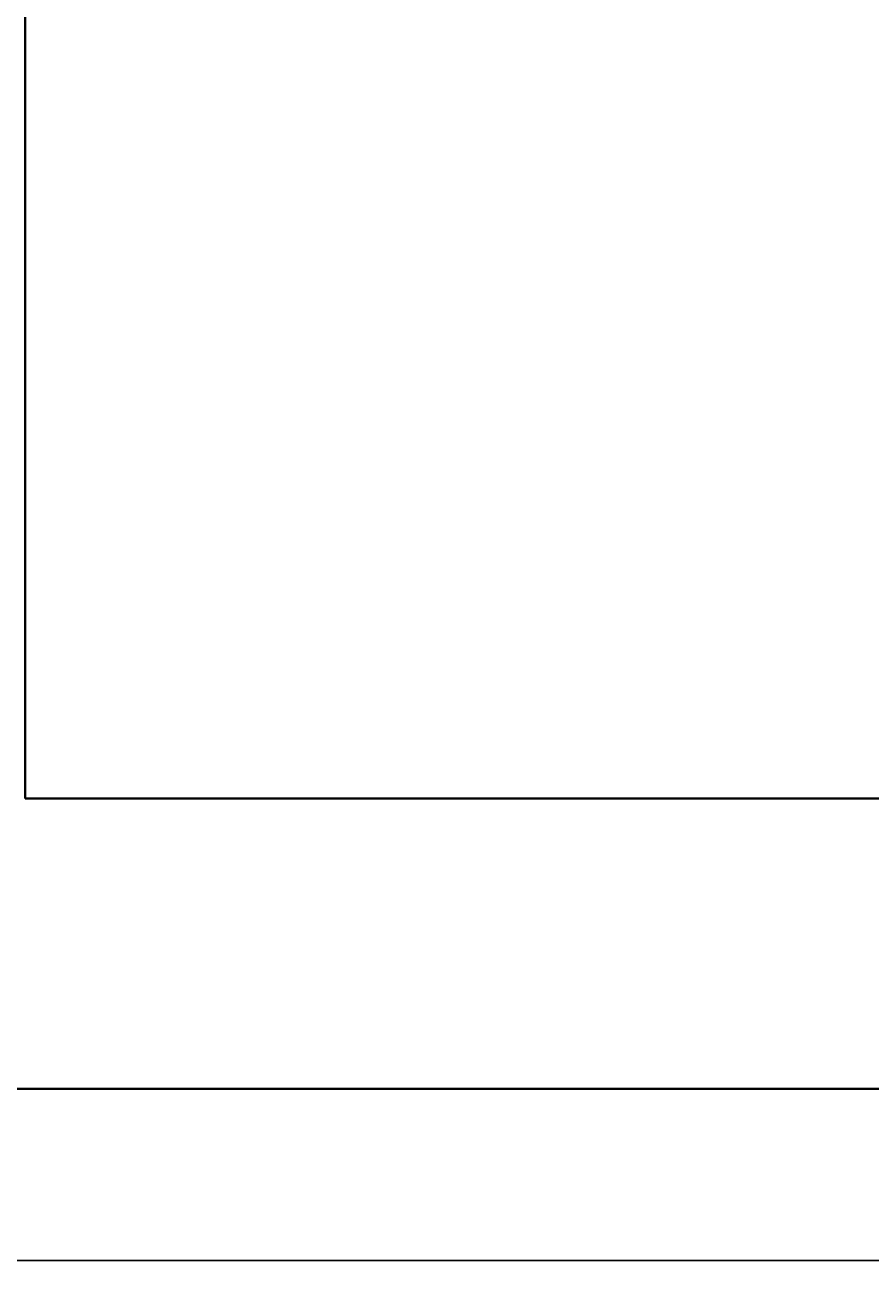
# Model space of a CAD drawing. Units: inches. Extents: x -61 to 1599, y -1316 to 257.
# Tile 45 of 204: x 88 to 114, y -447 to -408. Entities that reach past the tile are written whole.
import ezdxf

# ---------------------------------------------------------------- set-up
doc = ezdxf.new("R2010")
doc.units = ezdxf.units.IN
doc.header["$MEASUREMENT"] = 0
doc.layers.add('A-ANNO-DIMS', color=2, linetype='Continuous', lineweight=18)
doc.layers.add('WALLS', color=4, linetype='Continuous', lineweight=35)
doc.styles.get("Standard").update_dxf_attribs({"font": 'arial.ttf'})
doc.dimstyles.get("Standard").update_dxf_attribs({"dimtxt": 0.18, "dimasz": 0.18, "dimexe": 0.18, "dimexo": 0.0625, "dimgap": 0.09, "dimtad": 0, "dimtih": 1, "dimtoh": 1, "dimdec": 0, "dimzin": 0, "dimdsep": 46, "dimlunit": 3, "dimtxsty": 'Standard', "dimcen": 0.09, "dimadec": 0, "dimazin": 0, "dimtfac": 1, "dimtdec": 0, "dimtofl": 0, "dimtmove": 0, "dimatfit": 3, "dimfxl": 1, "dimtolj": 1, "dimtzin": 0, "dimarcsym": 0})

# ---------------------------------------------------------------- blocks, each defined once
blk = doc.blocks.new('*D687')
at = {"layer": 'A-ANNO-DIMS', "color": 0, "lineweight": -2, "transparency": 16777216}
for p, q in [((289.418, 181.677), (-61.077, 181.677)), ((-60.897, 181.497), (-60.897, -528.952)), ((-60.897, -1239.765), (-60.897, -529.316)), ((319.64, -1239.945), (-61.077, -1239.945))]:
    blk.add_line(p, q, dxfattribs=at)
at = {"layer": 'A-ANNO-DIMS', "color": 0, "transparency": 16777216}
for points in [[(-60.927, 181.497), (-60.867, 181.497), (-60.897, 181.677)], [(-60.927, -1239.765), (-60.867, -1239.765), (-60.897, -1239.945)]]:
    blk.add_solid(points, dxfattribs=at)
at = {"layer": 'DEFPOINTS', "color": 0, "transparency": 16777216}
for p in [(289.481, 181.677), (-60.897, -1239.945), (319.703, -1239.945)]:
    blk.add_point(p, dxfattribs=at)
at = {"layer": 'A-ANNO-DIMS', "color": 0, "transparency": 16777216, "insert": (-60.897, -529.134), "char_height": 0.18, "attachment_point": 5}
blk.add_mtext('\\A1;1421.6', dxfattribs=at)
blk = doc.blocks.new('*D699')
at = {"layer": 'A-ANNO-DIMS', "color": 0, "lineweight": -2, "transparency": 16777216}
for p, q in [((835.64, -167.169), (-61.077, -167.169)), ((-60.897, -167.349), (-60.897, -306.726)), ((-60.897, -446.466), (-60.897, -307.09)), ((841.64, -446.646), (-61.077, -446.646))]:
    blk.add_line(p, q, dxfattribs=at)
at = {"layer": 'A-ANNO-DIMS', "color": 0, "transparency": 16777216}
for points in [[(-60.927, -167.349), (-60.867, -167.349), (-60.897, -167.169)], [(-60.927, -446.466), (-60.867, -446.466), (-60.897, -446.646)]]:
    blk.add_solid(points, dxfattribs=at)
at = {"layer": 'DEFPOINTS', "color": 0, "transparency": 16777216}
for p in [(835.703, -167.169), (-60.897, -446.646), (841.703, -446.646)]:
    blk.add_point(p, dxfattribs=at)
at = {"layer": 'A-ANNO-DIMS', "color": 0, "transparency": 16777216, "insert": (-60.897, -306.908), "char_height": 0.18, "attachment_point": 5}
blk.add_mtext('\\A1;279.5', dxfattribs=at)
blk = doc.blocks.new('*D700')
at = {"layer": 'A-ANNO-DIMS', "color": 0, "lineweight": -2, "transparency": 16777216}
for p, q in [((14.703, -616.882), (14.703, 257.457)), ((179.752, -616.882), (179.752, 257.457)), ((14.883, 257.277), (96.772, 257.277)), ((179.572, 257.277), (97.683, 257.277))]:
    blk.add_line(p, q, dxfattribs=at)
at = {"layer": 'A-ANNO-DIMS', "color": 0, "transparency": 16777216}
for points in [[(14.883, 257.307), (14.883, 257.247), (14.703, 257.277)], [(179.572, 257.307), (179.572, 257.247), (179.752, 257.277)]]:
    blk.add_solid(points, dxfattribs=at)
at = {"layer": 'DEFPOINTS', "color": 0, "transparency": 16777216}
for p in [(179.752, 257.277), (14.703, -616.945), (179.752, -616.945)]:
    blk.add_point(p, dxfattribs=at)
at = {"layer": 'A-ANNO-DIMS', "color": 0, "transparency": 16777216, "insert": (97.227, 257.277), "char_height": 0.18, "attachment_point": 5}
blk.add_mtext('\\A1;165.05', dxfattribs=at)

msp = doc.modelspace()

# ---------------------------------------------------------------- linework, layer by layer
at = {"layer": 'WALLS'}
for p, q in [((87.7028, -288.3229), (87.7028, -432.3229)), ((87.7028, -432.3229), (237.7028, -432.3229)), ((14.7028, -441.3229), (237.7028, -441.3229))]:
    msp.add_line(p, q, dxfattribs=at)

# ---------------------------------------------------------------- dimensions: what is measured, and where the dimension line sits
at = {"layer": 'A-ANNO-DIMS'}
dim = msp.add_linear_dim(base=(179.7521, 257.2771), p1=(14.7028, -616.9446), p2=(179.7521, -616.9446), dimstyle='Standard', override={"dimdec": 2, "dimlfac": 1, "dimrnd": 0, "dimzin": 0, "dimdsep": 46, "dimlunit": 2}, dxfattribs=at)
dim.commit()
dim.dimension.update_dxf_attribs({"geometry": '*D700', "text_midpoint": (97.2274, 257.2771)})
for base, p1, p2, picture, middle in [((-60.8972, -1239.9446), (289.4807, 181.6771), (319.7028, -1239.9446), '*D687', (-60.8972, -529.1337)), ((-60.8972, -446.6462), (835.7028, -167.169), (841.7028, -446.6462), '*D699', (-60.8972, -306.9076))]:
    dim = msp.add_linear_dim(base=base, p1=p1, p2=p2, angle=90, dimstyle='Standard', override={"dimdec": 1, "dimlfac": 1, "dimrnd": 0, "dimzin": 0, "dimdsep": 46, "dimlunit": 2}, dxfattribs=at)
    dim.commit()
    dim.dimension.update_dxf_attribs({"geometry": picture, "text_midpoint": middle})

doc.saveas('drawing.dxf')
